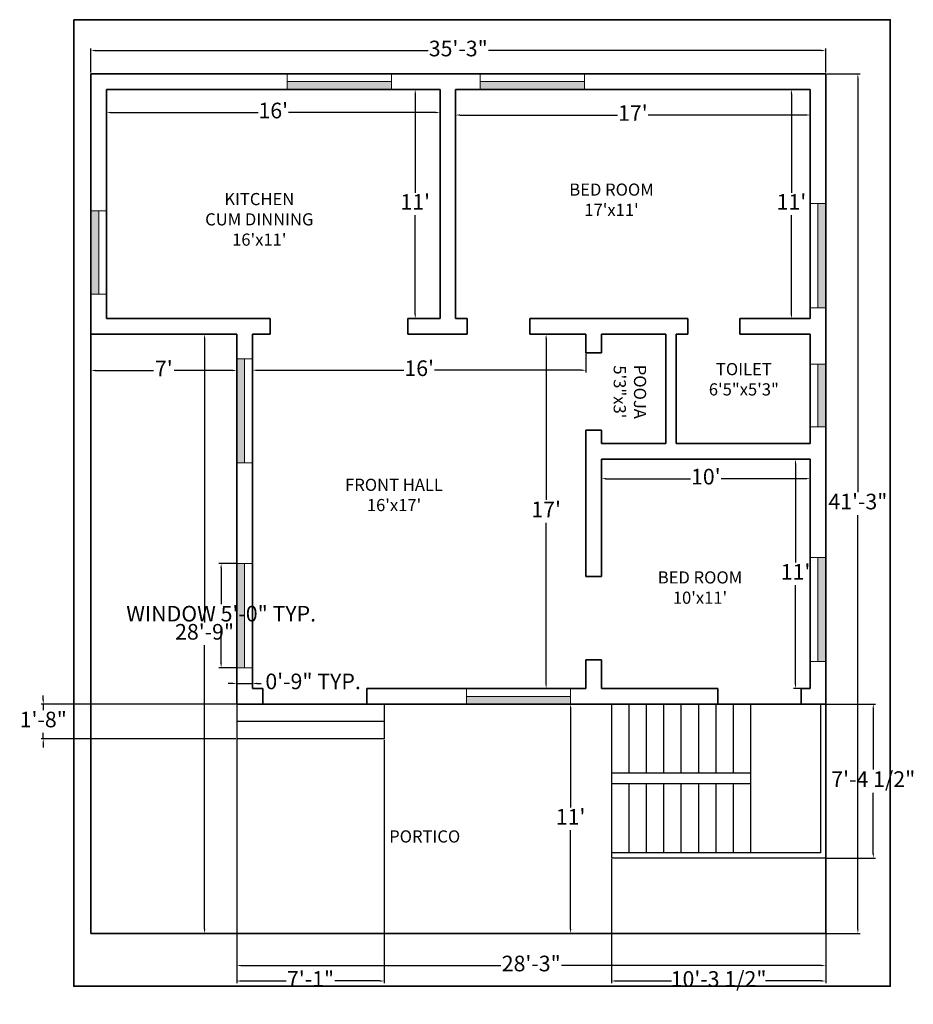
# Model space of a CAD drawing. Units: inches. Extents: x 1215 to 1730, y 1453 to 2020.
import ezdxf

# ---------------------------------------------------------------- set-up
doc = ezdxf.new("R2010")
doc.units = ezdxf.units.IN
for name, color, linetype, lineweight in [('A-ANNO-DIMS', 2, 'Continuous', 18), ('A-ANNO-TTLB', 7, 'Continuous', 35), ('A-AREA-IDEN', 7, 'Continuous', 25), ('A-FLOR-OTLN', 7, 'Continuous', 35), ('A-FLOR-STRS', 7, 'Continuous', 25), ('A-GLAZ', 4, 'Continuous', 18), ('A-WALL', 7, 'Continuous', 35)]:
    doc.layers.add(name, color=color, linetype=linetype, lineweight=lineweight)
doc.layers.add('A-GLAZ-PATT', color=18, linetype='Continuous', lineweight=13, true_color=0x000000)
doc.styles.get("Standard").update_dxf_attribs({"font": 'times.ttf'})
doc.dimstyles.new('ISO-25', dxfattribs={"dimtxt": 9, "dimasz": 2.5, "dimexe": 1.25, "dimexo": 0.625, "dimgap": 2, "dimtad": 0, "dimtih": 1, "dimtoh": 1, "dimdec": 1, "dimlunit": 4, "dimtxsty": 'Standard', "dimcen": 2.5, "dimadec": 0, "dimazin": 0, "dimtfac": 0.5, "dimtdec": 1, "dimtmove": 0, "dimatfit": 3, "dimfxl": 1, "dimarcsym": 0})

# ---------------------------------------------------------------- blocks, each defined once
blk = doc.blocks.new('*D1')
at = {"layer": 'A-ANNO-DIMS', "color": 0, "lineweight": -2, "transparency": 16777216}
for p, q in [((1265.3, 1979.14), (1265.3, 1965.17)), ((1457.3, 1979.14), (1457.3, 1965.17)), ((1267.8, 1966.42), (1352.52, 1966.42)), ((1454.8, 1966.42), (1370.08, 1966.42))]:
    blk.add_line(p, q, dxfattribs=at)
at = {"layer": 'A-ANNO-DIMS', "color": 0, "transparency": 16777216}
for points in [[(1267.8, 1966.84), (1267.8, 1966), (1265.3, 1966.42)], [(1454.8, 1966.84), (1454.8, 1966), (1457.3, 1966.42)]]:
    blk.add_solid(points, dxfattribs=at)
at = {"layer": 'Defpoints', "color": 0, "transparency": 16777216}
for p in [(1265.3, 1979.77), (1457.3, 1979.77), (1457.3, 1966.42)]:
    blk.add_point(p, dxfattribs=at)
at = {"layer": 'A-ANNO-DIMS', "color": 0, "transparency": 16777216, "insert": (1361.3, 1966.42), "char_height": 9, "attachment_point": 5}
blk.add_mtext("16'", dxfattribs=at)
blk = doc.blocks.new('*D2')
at = {"layer": 'A-ANNO-DIMS', "color": 0, "lineweight": -2, "transparency": 16777216}
for p, q in [((1456.67, 1979.77), (1441.78, 1979.77)), ((1443.03, 1977.27), (1443.03, 1920.27)), ((1443.03, 1850.27), (1443.03, 1907.27)), ((1456.67, 1847.77), (1441.78, 1847.77))]:
    blk.add_line(p, q, dxfattribs=at)
at = {"layer": 'A-ANNO-DIMS', "color": 0, "transparency": 16777216}
for points in [[(1442.61, 1977.27), (1443.45, 1977.27), (1443.03, 1979.77)], [(1442.61, 1850.27), (1443.45, 1850.27), (1443.03, 1847.77)]]:
    blk.add_solid(points, dxfattribs=at)
at = {"layer": 'Defpoints', "color": 0, "transparency": 16777216}
for p in [(1443.03, 1979.77), (1457.3, 1979.77), (1457.3, 1847.77)]:
    blk.add_point(p, dxfattribs=at)
at = {"layer": 'A-ANNO-DIMS', "color": 0, "transparency": 16777216, "insert": (1443.03, 1913.77), "char_height": 9, "attachment_point": 5}
blk.add_mtext("11'", dxfattribs=at)
blk = doc.blocks.new('*D3')
at = {"layer": 'A-ANNO-DIMS', "color": 0, "lineweight": -2, "transparency": 16777216}
for p, q in [((1466.3, 1979.14), (1466.3, 1963.74)), ((1670.3, 1979.14), (1670.3, 1963.74)), ((1468.8, 1964.99), (1559.52, 1964.99)), ((1667.8, 1964.99), (1577.08, 1964.99))]:
    blk.add_line(p, q, dxfattribs=at)
at = {"layer": 'A-ANNO-DIMS', "color": 0, "transparency": 16777216}
for points in [[(1468.8, 1965.41), (1468.8, 1964.57), (1466.3, 1964.99)], [(1667.8, 1965.41), (1667.8, 1964.57), (1670.3, 1964.99)]]:
    blk.add_solid(points, dxfattribs=at)
at = {"layer": 'Defpoints', "color": 0, "transparency": 16777216}
for p in [(1466.3, 1979.77), (1670.3, 1979.77), (1670.3, 1964.99)]:
    blk.add_point(p, dxfattribs=at)
at = {"layer": 'A-ANNO-DIMS', "color": 0, "transparency": 16777216, "insert": (1568.3, 1964.99), "char_height": 9, "attachment_point": 5}
blk.add_mtext("17'", dxfattribs=at)
blk = doc.blocks.new('*D4')
at = {"layer": 'A-ANNO-DIMS', "color": 0, "lineweight": -2, "transparency": 16777216}
for p, q in [((1669.67, 1979.77), (1658.3, 1979.77)), ((1659.55, 1977.27), (1659.55, 1920.27)), ((1659.55, 1850.27), (1659.55, 1907.27)), ((1669.67, 1847.77), (1658.3, 1847.77))]:
    blk.add_line(p, q, dxfattribs=at)
at = {"layer": 'A-ANNO-DIMS', "color": 0, "transparency": 16777216}
for points in [[(1659.13, 1977.27), (1659.97, 1977.27), (1659.55, 1979.77)], [(1659.13, 1850.27), (1659.97, 1850.27), (1659.55, 1847.77)]]:
    blk.add_solid(points, dxfattribs=at)
at = {"layer": 'Defpoints', "color": 0, "transparency": 16777216}
for p in [(1659.55, 1979.77), (1670.3, 1979.77), (1670.3, 1847.77)]:
    blk.add_point(p, dxfattribs=at)
at = {"layer": 'A-ANNO-DIMS', "color": 0, "transparency": 16777216, "insert": (1659.55, 1913.77), "char_height": 9, "attachment_point": 5}
blk.add_mtext("11'", dxfattribs=at)
blk = doc.blocks.new('*D5')
at = {"layer": 'A-ANNO-DIMS', "color": 0, "lineweight": -2, "transparency": 16777216}
for p, q in [((1669.67, 1766.77), (1660.69, 1766.77)), ((1661.94, 1764.27), (1661.94, 1707.27)), ((1661.94, 1637.27), (1661.94, 1694.27)), ((1669.67, 1634.77), (1660.69, 1634.77))]:
    blk.add_line(p, q, dxfattribs=at)
at = {"layer": 'A-ANNO-DIMS', "color": 0, "transparency": 16777216}
for points in [[(1661.52, 1764.27), (1662.35, 1764.27), (1661.94, 1766.77)], [(1661.52, 1637.27), (1662.35, 1637.27), (1661.94, 1634.77)]]:
    blk.add_solid(points, dxfattribs=at)
at = {"layer": 'Defpoints', "color": 0, "transparency": 16777216}
for p in [(1661.94, 1766.77), (1670.3, 1766.77), (1670.3, 1634.77)]:
    blk.add_point(p, dxfattribs=at)
at = {"layer": 'A-ANNO-DIMS', "color": 0, "transparency": 16777216, "insert": (1661.94, 1700.77), "char_height": 9, "attachment_point": 5}
blk.add_mtext("11'", dxfattribs=at)
blk = doc.blocks.new('*D6')
at = {"layer": 'A-ANNO-DIMS', "color": 0, "lineweight": -2, "transparency": 16777216}
for p, q in [((1550.3, 1766.14), (1550.3, 1754.36)), ((1670.3, 1766.14), (1670.3, 1754.36)), ((1552.8, 1755.61), (1601.52, 1755.61)), ((1667.8, 1755.61), (1619.08, 1755.61))]:
    blk.add_line(p, q, dxfattribs=at)
at = {"layer": 'A-ANNO-DIMS', "color": 0, "transparency": 16777216}
for points in [[(1552.8, 1756.03), (1552.8, 1755.2), (1550.3, 1755.61)], [(1667.8, 1756.03), (1667.8, 1755.2), (1670.3, 1755.61)]]:
    blk.add_solid(points, dxfattribs=at)
at = {"layer": 'Defpoints', "color": 0, "transparency": 16777216}
for p in [(1550.3, 1766.77), (1670.3, 1766.77), (1670.3, 1755.61)]:
    blk.add_point(p, dxfattribs=at)
at = {"layer": 'A-ANNO-DIMS', "color": 0, "transparency": 16777216, "insert": (1610.3, 1755.61), "char_height": 9, "attachment_point": 5}
blk.add_mtext("10'", dxfattribs=at)
blk = doc.blocks.new('*D7')
at = {"layer": 'A-ANNO-DIMS', "color": 0, "lineweight": -2, "transparency": 16777216}
for p, q in [((1540.67, 1838.77), (1517.14, 1838.77)), ((1518.39, 1836.27), (1518.39, 1743.36)), ((1518.39, 1637.27), (1518.39, 1730.18)), ((1540.67, 1634.77), (1517.14, 1634.77))]:
    blk.add_line(p, q, dxfattribs=at)
at = {"layer": 'A-ANNO-DIMS', "color": 0, "transparency": 16777216}
for points in [[(1517.97, 1836.27), (1518.8, 1836.27), (1518.39, 1838.77)], [(1517.97, 1637.27), (1518.8, 1637.27), (1518.39, 1634.77)]]:
    blk.add_solid(points, dxfattribs=at)
at = {"layer": 'Defpoints', "color": 0, "transparency": 16777216}
for p in [(1518.39, 1838.77), (1541.3, 1838.77), (1541.3, 1634.77)]:
    blk.add_point(p, dxfattribs=at)
at = {"layer": 'A-ANNO-DIMS', "color": 0, "transparency": 16777216, "insert": (1518.39, 1736.77), "char_height": 9, "attachment_point": 5}
blk.add_mtext("17'", dxfattribs=at)
blk = doc.blocks.new('*D8')
at = {"layer": 'A-ANNO-DIMS', "color": 0, "lineweight": -2, "transparency": 16777216}
for p, q in [((1349.3, 1827.48), (1349.3, 1816.8)), ((1541.3, 1827.48), (1541.3, 1816.8)), ((1351.8, 1818.05), (1436.52, 1818.05)), ((1538.8, 1818.05), (1454.08, 1818.05))]:
    blk.add_line(p, q, dxfattribs=at)
at = {"layer": 'A-ANNO-DIMS', "color": 0, "transparency": 16777216}
for points in [[(1351.8, 1818.47), (1351.8, 1817.63), (1349.3, 1818.05)], [(1538.8, 1818.47), (1538.8, 1817.63), (1541.3, 1818.05)]]:
    blk.add_solid(points, dxfattribs=at)
at = {"layer": 'Defpoints', "color": 0, "transparency": 16777216}
for p in [(1349.3, 1828.11), (1541.3, 1828.11), (1349.3, 1818.05)]:
    blk.add_point(p, dxfattribs=at)
at = {"layer": 'A-ANNO-DIMS', "color": 0, "transparency": 16777216, "insert": (1445.3, 1818.05), "char_height": 9, "attachment_point": 5}
blk.add_mtext("16'", dxfattribs=at)
blk = doc.blocks.new('*D9')
at = {"layer": 'A-ANNO-DIMS', "color": 0, "lineweight": -2, "transparency": 16777216}
for p, q in [((1256.3, 1838.14), (1256.3, 1816.65)), ((1340.3, 1838.14), (1340.3, 1816.65)), ((1258.8, 1817.9), (1292.31, 1817.9)), ((1337.8, 1817.9), (1304.29, 1817.9))]:
    blk.add_line(p, q, dxfattribs=at)
at = {"layer": 'A-ANNO-DIMS', "color": 0, "transparency": 16777216}
for points in [[(1258.8, 1818.32), (1258.8, 1817.49), (1256.3, 1817.9)], [(1337.8, 1818.32), (1337.8, 1817.49), (1340.3, 1817.9)]]:
    blk.add_solid(points, dxfattribs=at)
at = {"layer": 'Defpoints', "color": 0, "transparency": 16777216}
for p in [(1256.3, 1838.77), (1340.3, 1838.77), (1340.3, 1817.9)]:
    blk.add_point(p, dxfattribs=at)
at = {"layer": 'A-ANNO-DIMS', "color": 0, "transparency": 16777216, "insert": (1298.3, 1817.9), "char_height": 9, "attachment_point": 5}
blk.add_mtext("7'", dxfattribs=at)
blk = doc.blocks.new('*D10')
at = {"layer": 'A-ANNO-DIMS', "color": 0, "lineweight": -2, "transparency": 16777216}
for p, q in [((1256.92, 1838.77), (1323.01, 1838.77)), ((1321.76, 1836.27), (1321.76, 1672.86)), ((1321.76, 1496.27), (1321.76, 1659.68)), ((1256.92, 1493.77), (1323.01, 1493.77))]:
    blk.add_line(p, q, dxfattribs=at)
at = {"layer": 'A-ANNO-DIMS', "color": 0, "transparency": 16777216}
for points in [[(1321.35, 1836.27), (1322.18, 1836.27), (1321.76, 1838.77)], [(1321.35, 1496.27), (1322.18, 1496.27), (1321.76, 1493.77)]]:
    blk.add_solid(points, dxfattribs=at)
at = {"layer": 'Defpoints', "color": 0, "transparency": 16777216}
for p in [(1256.3, 1838.77), (1321.76, 1838.77), (1256.3, 1493.77)]:
    blk.add_point(p, dxfattribs=at)
at = {"layer": 'A-ANNO-DIMS', "color": 0, "transparency": 16777216, "insert": (1321.76, 1666.27), "char_height": 9, "attachment_point": 5}
blk.add_mtext('28\'-9"', dxfattribs=at)
blk = doc.blocks.new('*D11')
at = {"layer": 'A-ANNO-DIMS', "color": 0, "lineweight": -2, "transparency": 16777216}
for p, q in [((1678.67, 1625.77), (1531.22, 1625.77)), ((1532.47, 1623.27), (1532.47, 1566.27)), ((1532.47, 1496.27), (1532.47, 1553.27)), ((1678.67, 1493.77), (1531.22, 1493.77))]:
    blk.add_line(p, q, dxfattribs=at)
at = {"layer": 'A-ANNO-DIMS', "color": 0, "transparency": 16777216}
for points in [[(1532.05, 1623.27), (1532.89, 1623.27), (1532.47, 1625.77)], [(1532.05, 1496.27), (1532.89, 1496.27), (1532.47, 1493.77)]]:
    blk.add_solid(points, dxfattribs=at)
at = {"layer": 'Defpoints', "color": 0, "transparency": 16777216}
for p in [(1532.47, 1625.77), (1679.3, 1625.77), (1679.3, 1493.77)]:
    blk.add_point(p, dxfattribs=at)
at = {"layer": 'A-ANNO-DIMS', "color": 0, "transparency": 16777216, "insert": (1532.47, 1559.77), "char_height": 9, "attachment_point": 5}
blk.add_mtext("11'", dxfattribs=at)
blk = doc.blocks.new('*D12')
at = {"layer": 'A-ANNO-DIMS', "color": 0, "lineweight": -2, "transparency": 16777216}
for p, q in [((1340.3, 1625.14), (1340.3, 1474.02)), ((1679.3, 1625.14), (1679.3, 1474.02)), ((1342.8, 1475.27), (1492.29, 1475.27)), ((1676.8, 1475.27), (1527.3, 1475.27))]:
    blk.add_line(p, q, dxfattribs=at)
at = {"layer": 'A-ANNO-DIMS', "color": 0, "transparency": 16777216}
for points in [[(1342.8, 1475.69), (1342.8, 1474.86), (1340.3, 1475.27)], [(1676.8, 1475.69), (1676.8, 1474.86), (1679.3, 1475.27)]]:
    blk.add_solid(points, dxfattribs=at)
at = {"layer": 'Defpoints', "color": 0, "transparency": 16777216}
for p in [(1340.3, 1625.77), (1679.3, 1625.77), (1679.3, 1475.27)]:
    blk.add_point(p, dxfattribs=at)
at = {"layer": 'A-ANNO-DIMS', "color": 0, "transparency": 16777216, "insert": (1509.8, 1475.27), "char_height": 9, "attachment_point": 5}
blk.add_mtext('28\'-3"', dxfattribs=at)
blk = doc.blocks.new('*D13')
at = {"layer": 'A-ANNO-DIMS', "color": 0, "lineweight": -2, "transparency": 16777216}
for p, q in [((1256.3, 1989.39), (1256.3, 2003.38)), ((1258.8, 2002.13), (1450.42, 2002.13)), ((1676.8, 2002.13), (1485.18, 2002.13)), ((1679.3, 1989.39), (1679.3, 2003.38))]:
    blk.add_line(p, q, dxfattribs=at)
at = {"layer": 'A-ANNO-DIMS', "color": 0, "transparency": 16777216}
for points in [[(1258.8, 2002.54), (1258.8, 2001.71), (1256.3, 2002.13)], [(1676.8, 2002.54), (1676.8, 2001.71), (1679.3, 2002.13)]]:
    blk.add_solid(points, dxfattribs=at)
at = {"layer": 'Defpoints', "color": 0, "transparency": 16777216}
for p in [(1679.3, 2002.13), (1256.3, 1988.77), (1679.3, 1988.77)]:
    blk.add_point(p, dxfattribs=at)
at = {"layer": 'A-ANNO-DIMS', "color": 0, "transparency": 16777216, "insert": (1467.8, 2002.13), "char_height": 9, "attachment_point": 5}
blk.add_mtext('35\'-3"', dxfattribs=at)
blk = doc.blocks.new('*D14')
at = {"layer": 'A-ANNO-DIMS', "color": 0, "lineweight": -2, "transparency": 16777216}
for p, q in [((1679.92, 1988.77), (1699.08, 1988.77)), ((1697.83, 1986.27), (1697.83, 1747.85)), ((1697.83, 1496.27), (1697.83, 1734.69)), ((1679.92, 1493.77), (1699.08, 1493.77))]:
    blk.add_line(p, q, dxfattribs=at)
at = {"layer": 'A-ANNO-DIMS', "color": 0, "transparency": 16777216}
for points in [[(1697.41, 1986.27), (1698.24, 1986.27), (1697.83, 1988.77)], [(1697.41, 1496.27), (1698.24, 1496.27), (1697.83, 1493.77)]]:
    blk.add_solid(points, dxfattribs=at)
at = {"layer": 'Defpoints', "color": 0, "transparency": 16777216}
for p in [(1679.3, 1988.77), (1679.3, 1493.77), (1697.83, 1493.77)]:
    blk.add_point(p, dxfattribs=at)
at = {"layer": 'A-ANNO-DIMS', "color": 0, "transparency": 16777216, "insert": (1697.83, 1741.27), "char_height": 9, "attachment_point": 5}
blk.add_mtext('41\'-3"', dxfattribs=at)
blk = doc.blocks.new('WIN-60IN')
for p, q in [((0, 9), (0, 0)), ((60, 9), (60, 0)), ((60, 4.5), (0, 4.5))]:
    blk.add_line(p, q)
blk = doc.blocks.new('*D16')
at = {"layer": 'A-ANNO-DIMS', "color": 0, "lineweight": -2, "transparency": 16777216}
for p, q in [((1339.67, 1706.71), (1330.05, 1706.71)), ((1331.3, 1704.21), (1331.3, 1683.31)), ((1331.3, 1649.21), (1331.3, 1670.11)), ((1339.67, 1646.71), (1330.05, 1646.71))]:
    blk.add_line(p, q, dxfattribs=at)
at = {"layer": 'A-ANNO-DIMS', "color": 0, "transparency": 16777216}
for points in [[(1330.88, 1704.21), (1331.71, 1704.21), (1331.3, 1706.71)], [(1330.88, 1649.21), (1331.71, 1649.21), (1331.3, 1646.71)]]:
    blk.add_solid(points, dxfattribs=at)
at = {"layer": 'Defpoints', "color": 0, "transparency": 16777216}
for p in [(1340.3, 1706.71), (1331.3, 1646.71), (1340.3, 1646.71)]:
    blk.add_point(p, dxfattribs=at)
at = {"layer": 'A-ANNO-DIMS', "color": 0, "transparency": 16777216, "insert": (1331.3, 1676.71), "char_height": 9, "attachment_point": 5}
blk.add_mtext('WINDOW 5\'-0" TYP.', dxfattribs=at)
blk = doc.blocks.new('*D17')
at = {"layer": 'A-ANNO-DIMS', "color": 0, "lineweight": -2, "transparency": 16777216}
for p, q in [((1340.3, 1646.08), (1340.3, 1636.46)), ((1349.3, 1646.08), (1349.3, 1636.46)), ((1337.8, 1637.71), (1335.3, 1637.71)), ((1340.3, 1637.71), (1349.3, 1637.71)), ((1351.8, 1637.71), (1354.3, 1637.71))]:
    blk.add_line(p, q, dxfattribs=at)
at = {"layer": 'A-ANNO-DIMS', "color": 0, "transparency": 16777216}
for points in [[(1337.8, 1638.12), (1337.8, 1637.29), (1340.3, 1637.71)], [(1351.8, 1638.12), (1351.8, 1637.29), (1349.3, 1637.71)]]:
    blk.add_solid(points, dxfattribs=at)
at = {"layer": 'Defpoints', "color": 0, "transparency": 16777216}
for p in [(1340.3, 1646.71), (1349.3, 1646.71), (1349.3, 1637.71)]:
    blk.add_point(p, dxfattribs=at)
at = {"layer": 'A-ANNO-DIMS', "color": 0, "transparency": 16777216, "insert": (1384.23, 1637.71), "char_height": 9, "attachment_point": 5}
blk.add_mtext('0\'-9" TYP.', dxfattribs=at)
blk = doc.blocks.new('*D18')
at = {"layer": 'A-ANNO-DIMS', "color": 0, "lineweight": -2, "transparency": 16777216}
for p, q in [((1556.01, 1536.53), (1556.01, 1465.12)), ((1679.3, 1536.53), (1679.3, 1465.12)), ((1558.51, 1466.37), (1590.63, 1466.37)), ((1676.8, 1466.37), (1644.67, 1466.37))]:
    blk.add_line(p, q, dxfattribs=at)
at = {"layer": 'A-ANNO-DIMS', "color": 0, "transparency": 16777216}
for points in [[(1558.51, 1466.79), (1558.51, 1465.95), (1556.01, 1466.37)], [(1676.8, 1466.79), (1676.8, 1465.95), (1679.3, 1466.37)]]:
    blk.add_solid(points, dxfattribs=at)
at = {"layer": 'Defpoints', "color": 0, "transparency": 16777216}
for p in [(1556.01, 1537.15), (1679.3, 1537.15), (1679.3, 1466.37)]:
    blk.add_point(p, dxfattribs=at)
at = {"layer": 'A-ANNO-DIMS', "color": 0, "transparency": 16777216, "insert": (1617.65, 1466.37), "char_height": 9, "attachment_point": 5}
blk.add_mtext('10\'-3 1/2"', dxfattribs=at)
blk = doc.blocks.new('*D19')
at = {"layer": 'A-ANNO-DIMS', "color": 0, "lineweight": -2, "transparency": 16777216}
for p, q in [((1679.92, 1625.77), (1707.95, 1625.77)), ((1706.7, 1623.27), (1706.7, 1588.17)), ((1706.7, 1539.65), (1706.7, 1574.76)), ((1679.92, 1537.15), (1707.95, 1537.15))]:
    blk.add_line(p, q, dxfattribs=at)
at = {"layer": 'A-ANNO-DIMS', "color": 0, "transparency": 16777216}
for points in [[(1706.28, 1623.27), (1707.11, 1623.27), (1706.7, 1625.77)], [(1706.28, 1539.65), (1707.11, 1539.65), (1706.7, 1537.15)]]:
    blk.add_solid(points, dxfattribs=at)
at = {"layer": 'Defpoints', "color": 0, "transparency": 16777216}
for p in [(1679.3, 1625.77), (1706.7, 1625.77), (1679.3, 1537.15)]:
    blk.add_point(p, dxfattribs=at)
at = {"layer": 'A-ANNO-DIMS', "color": 0, "transparency": 16777216, "insert": (1706.7, 1581.46), "char_height": 9, "attachment_point": 5}
blk.add_mtext('7\'-4 1/2"', dxfattribs=at)
blk = doc.blocks.new('*D20')
at = {"layer": 'A-ANNO-DIMS', "color": 0, "lineweight": -2, "transparency": 16777216}
for p, q in [((1340.3, 1605.14), (1340.3, 1465.12)), ((1425.21, 1605.14), (1425.21, 1465.12)), ((1342.8, 1466.37), (1368.68, 1466.37)), ((1422.71, 1466.37), (1396.83, 1466.37))]:
    blk.add_line(p, q, dxfattribs=at)
at = {"layer": 'A-ANNO-DIMS', "color": 0, "transparency": 16777216}
for points in [[(1342.8, 1466.79), (1342.8, 1465.95), (1340.3, 1466.37)], [(1422.71, 1466.79), (1422.71, 1465.95), (1425.21, 1466.37)]]:
    blk.add_solid(points, dxfattribs=at)
at = {"layer": 'Defpoints', "color": 0, "transparency": 16777216}
for p in [(1340.3, 1605.77), (1425.21, 1605.77), (1425.21, 1466.37)]:
    blk.add_point(p, dxfattribs=at)
at = {"layer": 'A-ANNO-DIMS', "color": 0, "transparency": 16777216, "insert": (1382.75, 1466.37), "char_height": 9, "attachment_point": 5}
blk.add_mtext('7\'-1"', dxfattribs=at)
blk = doc.blocks.new('*D21')
at = {"layer": 'A-ANNO-DIMS', "color": 0, "lineweight": -2, "transparency": 16777216}
for p, q in [((1228.9, 1628.27), (1228.9, 1630.77)), ((1339.67, 1625.77), (1227.65, 1625.77)), ((1228.9, 1625.77), (1228.9, 1622.35)), ((1339.67, 1605.77), (1227.65, 1605.77)), ((1228.9, 1605.77), (1228.9, 1609.19)), ((1228.9, 1603.27), (1228.9, 1600.77))]:
    blk.add_line(p, q, dxfattribs=at)
at = {"layer": 'A-ANNO-DIMS', "color": 0, "transparency": 16777216}
for points in [[(1228.48, 1628.27), (1229.31, 1628.27), (1228.9, 1625.77)], [(1228.48, 1603.27), (1229.31, 1603.27), (1228.9, 1605.77)]]:
    blk.add_solid(points, dxfattribs=at)
at = {"layer": 'Defpoints', "color": 0, "transparency": 16777216}
for p in [(1228.9, 1625.77), (1340.3, 1625.77), (1340.3, 1605.77)]:
    blk.add_point(p, dxfattribs=at)
at = {"layer": 'A-ANNO-DIMS', "color": 0, "transparency": 16777216, "insert": (1228.9, 1615.77), "char_height": 9, "attachment_point": 5}
blk.add_mtext('1\'-8"', dxfattribs=at)

msp = doc.modelspace()

# ---------------------------------------------------------------- hatches: boundary and pattern name
at = {"layer": 'A-GLAZ-PATT'}
h = msp.add_hatch(color=256, dxfattribs=at)
h.dxf.hatch_style = 1
h.paths.add_polyline_path([(1429.27, 1984.27), (1369.27, 1984.27), (1369.27, 1979.77), (1429.27, 1979.77)])
h.paths.add_polyline_path([(1540.38, 1984.27), (1480.38, 1984.27), (1480.38, 1979.77), (1540.38, 1979.77)])
h.paths.add_polyline_path([(1679.3, 1914.07), (1674.8, 1914.07), (1674.8, 1854.07), (1679.3, 1854.07)])
h.paths.add_polyline_path([(1679.3, 1821.54), (1674.8, 1821.54), (1674.8, 1785.54), (1679.3, 1785.54)])
h.paths.add_polyline_path([(1344.8, 1824.65), (1340.3, 1824.65), (1340.3, 1764.65), (1344.8, 1764.65)])
h.paths.add_polyline_path([(1344.8, 1706.71), (1340.3, 1706.71), (1340.3, 1646.71), (1344.8, 1646.71)])
h.paths.add_polyline_path([(1679.3, 1710.26), (1674.8, 1710.26), (1674.8, 1650.26), (1679.3, 1650.26)])
h.paths.add_polyline_path([(1532.47, 1630.27), (1472.47, 1630.27), (1472.47, 1625.77), (1532.47, 1625.77)])
h = msp.add_hatch(color=256, dxfattribs=at)
h.dxf.hatch_style = 1
h.paths.add_polyline_path([(1260.8, 1909.88), (1256.3, 1909.88), (1256.3, 1861.88), (1260.8, 1861.88)])

# ---------------------------------------------------------------- linework, layer by layer
at = {"layer": 'A-ANNO-TTLB'}
msp.add_lwpolyline([(1246.44, 2019.89), (1716.48, 2019.89), (1716.48, 1463.3), (1246.44, 1463.3)], close=True, dxfattribs=at)
at = {"layer": 'A-FLOR-OTLN'}
for p, q in [((1256.3, 1988.77), (1679.3, 1988.77)), ((1256.3, 1493.77), (1256.3, 1988.77)), ((1679.3, 1988.77), (1679.3, 1493.77)), ((1679.3, 1493.77), (1256.3, 1493.77))]:
    msp.add_line(p, q, dxfattribs=at)
at = {"layer": 'A-FLOR-STRS'}
for p, q in [((1340.3, 1625.77), (1340.3, 1605.77)), ((1415.21, 1625.77), (1425.21, 1625.77)), ((1425.21, 1625.77), (1425.21, 1605.77)), ((1556.01, 1625.77), (1556.01, 1540.15)), ((1566.01, 1625.77), (1566.01, 1585.96)), ((1576.01, 1625.77), (1576.01, 1585.96)), ((1586.01, 1625.77), (1586.01, 1585.96)), ((1596.01, 1625.77), (1596.01, 1585.96)), ((1606.01, 1625.77), (1606.01, 1585.96)), ((1616.01, 1625.77), (1616.01, 1585.96)), ((1626.01, 1625.77), (1626.01, 1585.96)), ((1636.01, 1625.77), (1636.01, 1540.15)), ((1676.3, 1625.77), (1676.3, 1540.15)), ((1425.21, 1615.77), (1340.3, 1615.77)), ((1425.21, 1605.77), (1340.3, 1605.77)), ((1636.01, 1585.96), (1556.01, 1585.96)), ((1636.01, 1579.96), (1556.01, 1579.96)), ((1566.01, 1579.96), (1566.01, 1540.15)), ((1576.01, 1579.96), (1576.01, 1540.15)), ((1586.01, 1579.96), (1586.01, 1540.15)), ((1596.01, 1579.96), (1596.01, 1540.15)), ((1606.01, 1579.96), (1606.01, 1540.15)), ((1616.01, 1579.96), (1616.01, 1540.15)), ((1626.01, 1579.96), (1626.01, 1540.15)), ((1676.3, 1540.15), (1556.01, 1540.15)), ((1556.01, 1540.15), (1556.01, 1537.15)), ((1679.3, 1537.15), (1556.01, 1537.15))]:
    msp.add_line(p, q, dxfattribs=at)
at = {"layer": 'A-GLAZ'}
for p, q in [((1265.3, 1909.88), (1256.3, 1909.88)), ((1260.8, 1909.88), (1260.8, 1861.88)), ((1265.3, 1861.88), (1256.3, 1861.88)), ((1670.3, 1821.54), (1679.3, 1821.54)), ((1674.8, 1785.54), (1674.8, 1821.54)), ((1670.3, 1785.54), (1679.3, 1785.54))]:
    msp.add_line(p, q, dxfattribs=at)
at = {"layer": 'A-WALL'}
for p, q in [((1265.3, 1979.77), (1457.3, 1979.77)), ((1265.3, 1847.77), (1265.3, 1979.77)), ((1457.3, 1847.77), (1457.3, 1979.77)), ((1466.3, 1847.77), (1466.3, 1979.77)), ((1466.3, 1979.77), (1670.3, 1979.77)), ((1670.3, 1979.77), (1670.3, 1847.77)), ((1265.3, 1847.77), (1359.56, 1847.77)), ((1359.56, 1838.77), (1359.56, 1847.77)), ((1438.79, 1847.77), (1438.79, 1838.77)), ((1438.79, 1847.77), (1457.3, 1847.77)), ((1466.3, 1847.77), (1472.9, 1847.77)), ((1472.9, 1847.77), (1472.9, 1838.77)), ((1508.9, 1847.77), (1508.9, 1838.77)), ((1508.9, 1847.77), (1599.94, 1847.77)), ((1599.94, 1838.77), (1599.94, 1847.77)), ((1629.94, 1838.77), (1629.94, 1847.77)), ((1629.94, 1847.77), (1670.3, 1847.77)), ((1265.3, 1838.77), (1256.3, 1838.77)), ((1265.3, 1838.77), (1340.3, 1838.77)), ((1265.3, 1838.77), (1340.3, 1838.77)), ((1340.3, 1625.77), (1340.3, 1838.77)), ((1349.3, 1838.77), (1359.56, 1838.77)), ((1349.3, 1838.77), (1359.56, 1838.77)), ((1349.3, 1634.77), (1349.3, 1838.77)), ((1438.79, 1838.77), (1472.9, 1838.77)), ((1438.79, 1838.77), (1457.3, 1838.77)), ((1466.3, 1838.77), (1472.9, 1838.77)), ((1508.9, 1838.77), (1541.3, 1838.77)), ((1508.9, 1838.77), (1541.3, 1838.77)), ((1541.3, 1828.11), (1541.3, 1838.77)), ((1550.3, 1838.77), (1587.3, 1838.77)), ((1550.3, 1838.77), (1587.3, 1838.77)), ((1550.3, 1828.11), (1550.3, 1838.77)), ((1587.3, 1838.77), (1587.3, 1775.77)), ((1593.3, 1838.77), (1593.3, 1775.77)), ((1593.3, 1838.77), (1599.94, 1838.77)), ((1593.3, 1838.77), (1599.94, 1838.77)), ((1629.94, 1838.77), (1670.3, 1838.77)), ((1629.94, 1838.77), (1670.3, 1838.77)), ((1670.3, 1838.77), (1670.3, 1775.77)), ((1541.3, 1828.11), (1550.3, 1828.11)), ((1550.3, 1783.51), (1541.3, 1783.51)), ((1541.3, 1699.31), (1541.3, 1783.51)), ((1550.3, 1775.77), (1550.3, 1783.51)), ((1550.3, 1775.77), (1587.3, 1775.77)), ((1593.3, 1775.77), (1670.3, 1775.77)), ((1550.3, 1766.77), (1670.3, 1766.77)), ((1550.3, 1699.31), (1550.3, 1766.77)), ((1670.3, 1766.77), (1670.3, 1634.77)), ((1541.3, 1699.31), (1550.3, 1699.31)), ((1541.3, 1634.77), (1541.3, 1651.31)), ((1541.3, 1651.31), (1550.3, 1651.31)), ((1550.3, 1634.77), (1550.3, 1651.31)), ((1349.3, 1634.77), (1355.21, 1634.77)), ((1355.21, 1634.77), (1355.21, 1625.77)), ((1415.21, 1634.77), (1415.21, 1625.77)), ((1415.21, 1634.77), (1541.3, 1634.77)), ((1550.3, 1634.77), (1617.18, 1634.77)), ((1617.18, 1634.77), (1617.18, 1625.77)), ((1665.18, 1634.77), (1665.18, 1625.77)), ((1665.18, 1634.77), (1670.3, 1634.77)), ((1349.3, 1625.77), (1340.3, 1625.77)), ((1349.3, 1625.77), (1541.3, 1625.77)), ((1541.3, 1625.77), (1679.3, 1625.77))]:
    msp.add_line(p, q, dxfattribs=at)

# ---------------------------------------------------------------- block references
at = {"layer": 'A-GLAZ'}
for p in [(1369.27, 1979.77), (1472.47, 1625.77)]:
    msp.add_blockref('WIN-60IN', p, dxfattribs=at)
for p, rotation in [((1540.38, 1988.77), 180), ((1670.3, 1914.07), 270.0000000000025), ((1349.3, 1764.65), 90.00000000000044), ((1340.3, 1706.71), 270.0000000000017), ((1670.3, 1710.26), 270.0000000000009)]:
    msp.add_blockref('WIN-60IN', p, dxfattribs=dict(at, rotation=rotation))

# ---------------------------------------------------------------- texts
at = {"layer": 'A-AREA-IDEN', "char_height": 7, "attachment_point": 1}
for s, width, insert in [("\\pxqc;{\\fTimes New Roman|b1|i0|c0|p18;BED ROOM\\P17'x11'}", 146.6037, (1482.71, 1925.56)), ("\\pxqc;{\\fTimes New Roman|b1|i0|c0|p18;KITCHEN\\PCUM DINNING\\P16'x11'}", 129.448, (1288.54, 1920.1)), ('\\pxqc;{\\fTimes New Roman|b1|i0|c0|p18;TOILET\\P6\'5"x5\'3"}', 65.7692, (1599.31, 1822.19)), ("\\pxqc;{\\fTimes New Roman|b1|i0|c0|p18;FRONT HALL\\P16'x17'}", 130.2278, (1365.71, 1755.58)), ("\\pxqc;{\\fTimes New Roman|b1|i0|c0|p18;BED ROOM\\P10'x11'}", 89.8474, (1562.03, 1702.25)), ('\\pxqc;{\\fTimes New Roman|b1|i0|c0|p18;PORTICO}', 94.4315, (1401.26, 1553.11))]:
    msp.add_mtext_dynamic_manual_height_columns(s, width=width, gutter_width=12.5, heights=[0], dxfattribs=dict(at, insert=insert))
at = {"layer": 'A-AREA-IDEN', "insert": (1575.93, 1864.89), "char_height": 7, "attachment_point": 1, "rotation": 270}
msp.add_mtext_dynamic_manual_height_columns('\\pxqc;{\\fTimes New Roman|b1|i0|c0|p18;POOJA\\P5\'3"x3\'}', width=118.5682, gutter_width=12.5, heights=[0], dxfattribs=at)

# ---------------------------------------------------------------- dimensions: what is measured, and where the dimension line sits
at = {"layer": 'A-ANNO-DIMS'}
for base, p1, p2, override, picture, middle in [((1679.3, 2002.13), (1256.3, 1988.77), (1679.3, 1988.77), {"dimclrd": 0, "dimclre": 0, "dimclrt": 0}, '*D13', (1467.8, 2002.13)), ((1457.3, 1966.42), (1265.3, 1979.77), (1457.3, 1979.77), {"dimclrd": 0, "dimclre": 0, "dimclrt": 0}, '*D1', (1361.3, 1966.42)), ((1670.3, 1964.99), (1466.3, 1979.77), (1670.3, 1979.77), {"dimclrd": 0, "dimclre": 0, "dimclrt": 0}, '*D3', (1568.3, 1964.99)), ((1340.3, 1817.9), (1256.3, 1838.77), (1340.3, 1838.77), {"dimclrd": 0, "dimclre": 0, "dimclrt": 0}, '*D9', (1298.3, 1817.9)), ((1349.3, 1818.05), (1541.3, 1828.11), (1349.3, 1828.11), {"dimclrd": 0, "dimclre": 0, "dimclrt": 0}, '*D8', (1445.3, 1818.05)), ((1670.3, 1755.61), (1550.3, 1766.77), (1670.3, 1766.77), {"dimclrd": 0, "dimclre": 0, "dimclrt": 0}, '*D6', (1610.3, 1755.61)), ((1679.3, 1475.27), (1340.3, 1625.77), (1679.3, 1625.77), {"dimclrd": 0, "dimclre": 0, "dimclrt": 0}, '*D12', (1509.8, 1475.27)), ((1425.21, 1466.37), (1340.3, 1605.77), (1425.21, 1605.77), {"dimdec": 1, "dimlfac": 1, "dimrnd": 0, "dimzin": 1, "dimdsep": 46, "dimlunit": 4, "dimfrac": 2}, '*D20', (1382.75, 1466.37)), ((1679.3, 1466.37), (1556.01, 1537.15), (1679.3, 1537.15), {"dimdec": 1, "dimlfac": 1, "dimrnd": 0, "dimzin": 1, "dimdsep": 46, "dimlunit": 4, "dimfrac": 2}, '*D18', (1617.65, 1466.37))]:
    dim = msp.add_linear_dim(base=base, p1=p1, p2=p2, dimstyle='ISO-25', override=override, dxfattribs=at)
    dim.commit()
    dim.dimension.update_dxf_attribs({"geometry": picture, "text_midpoint": middle})
for base, p1, p2, override, picture, middle in [((1697.83, 1493.77), (1679.3, 1988.77), (1679.3, 1493.77), {"dimclrd": 0, "dimclre": 0, "dimclrt": 0}, '*D14', (1697.83, 1741.27)), ((1443.03, 1979.77), (1457.3, 1847.77), (1457.3, 1979.77), {"dimclrd": 0, "dimclre": 0, "dimclrt": 0}, '*D2', (1443.03, 1913.77)), ((1659.55, 1979.77), (1670.3, 1847.77), (1670.3, 1979.77), {"dimclrd": 0, "dimclre": 0, "dimclrt": 0}, '*D4', (1659.55, 1913.77)), ((1321.76, 1838.77), (1256.3, 1493.77), (1256.3, 1838.77), {"dimclrd": 0, "dimclre": 0, "dimclrt": 0}, '*D10', (1321.76, 1666.27)), ((1518.39, 1838.77), (1541.3, 1634.77), (1541.3, 1838.77), {"dimclrd": 0, "dimclre": 0, "dimclrt": 0}, '*D7', (1518.39, 1736.77)), ((1661.94, 1766.77), (1670.3, 1634.77), (1670.3, 1766.77), {"dimclrd": 0, "dimclre": 0, "dimclrt": 0}, '*D5', (1661.94, 1700.77)), ((1228.9, 1625.77), (1340.3, 1605.77), (1340.3, 1625.77), {"dimdec": 1, "dimlfac": 1, "dimrnd": 0, "dimzin": 1, "dimdsep": 46, "dimlunit": 4, "dimfrac": 2}, '*D21', (1228.9, 1615.77)), ((1532.47, 1625.77), (1679.3, 1493.77), (1679.3, 1625.77), {"dimclrd": 0, "dimclre": 0, "dimclrt": 0}, '*D11', (1532.47, 1559.77)), ((1706.7, 1625.77), (1679.3, 1537.15), (1679.3, 1625.77), {"dimdec": 1, "dimlfac": 1, "dimrnd": 0, "dimzin": 1, "dimdsep": 46, "dimlunit": 4, "dimfrac": 2}, '*D19', (1706.7, 1581.46))]:
    dim = msp.add_linear_dim(base=base, p1=p1, p2=p2, angle=90, dimstyle='ISO-25', override=override, dxfattribs=at)
    dim.commit()
    dim.dimension.update_dxf_attribs({"geometry": picture, "text_midpoint": middle})
for base, p1, p2, angle, text, picture, middle in [((1331.3, 1646.71), (1340.3, 1706.71), (1340.3, 1646.71), 270, 'WINDOW <> TYP.', '*D16', (1331.3, 1676.71)), ((1349.3, 1637.71), (1340.3, 1646.71), (1349.3, 1646.71), 0, '<> TYP.', '*D17', (1384.23, 1637.71))]:
    dim = msp.add_linear_dim(base=base, p1=p1, p2=p2, angle=angle, text=text, dimstyle='ISO-25', override={"dimdec": 1, "dimlfac": 1, "dimrnd": 0, "dimzin": 1, "dimdsep": 46, "dimlunit": 4, "dimfrac": 2}, dxfattribs=at)
    dim.commit()
    dim.dimension.update_dxf_attribs({"geometry": picture, "text_midpoint": middle})

doc.saveas('drawing.dxf')
